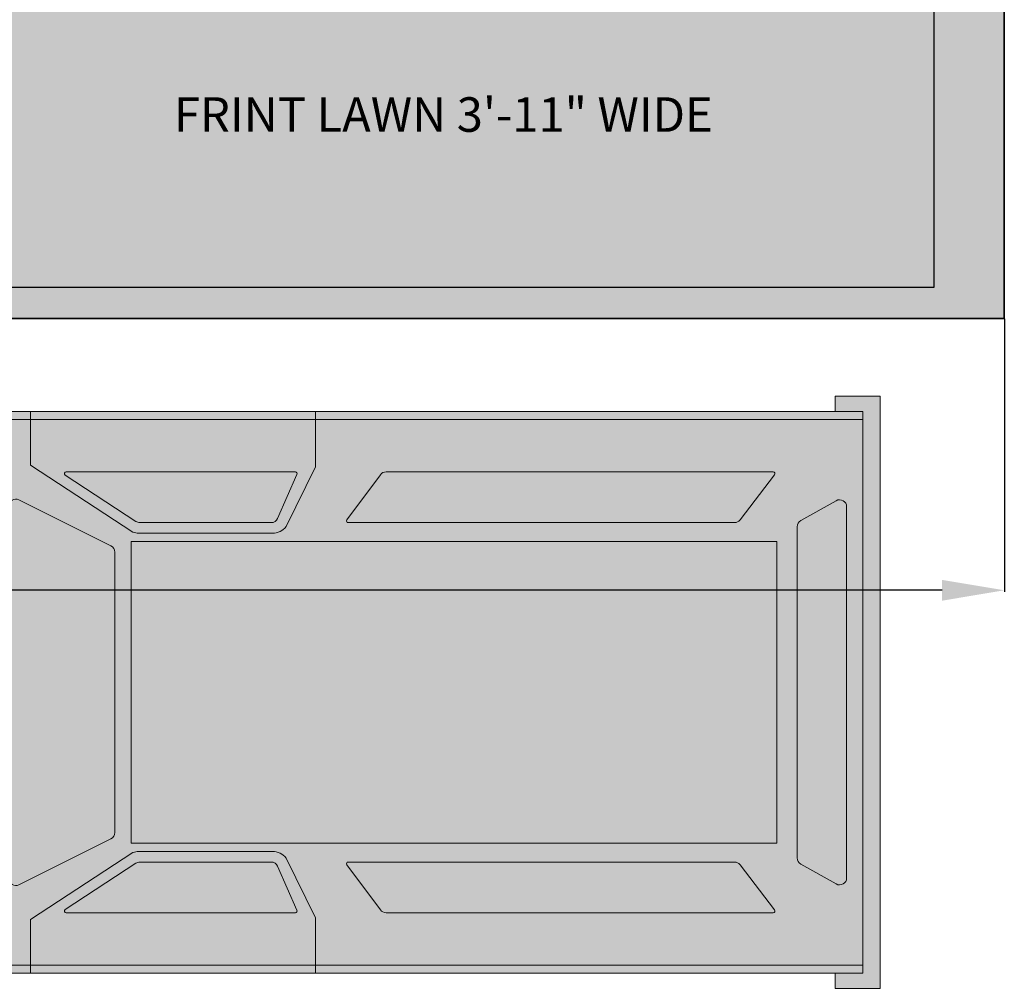
# Model space of a CAD drawing. Units: inches. Extents: x 389 to 971, y 148 to 870.
# Tile 5 of 14: x 722 to 848, y 148 to 273. Entities that reach past the tile are written whole.
import ezdxf

# ---------------------------------------------------------------- set-up
doc = ezdxf.new("R2010")
doc.units = ezdxf.units.IN
doc.header["$MEASUREMENT"] = 0
for name, color, linetype, lineweight in [('A-ANNO-DIMS', 2, 'Continuous', 18), ('A-ANNO-TEXT', 7, 'Continuous', 18), ('C-PROP', 7, 'Continuous', 35), ('C-VEHI', 8, 'Continuous', 13), ('L-GRND-BASE-PATT', 8, 'Continuous', 13), ('L-WALL', 7, 'Continuous', 30)]:
    doc.layers.add(name, color=color, linetype=linetype, lineweight=lineweight)
for name, color, linetype, lineweight, true_color in [('A-WALL-PATT', 18, 'Continuous', 13, 0x000000), ('C-VEHI-PATT', 18, 'Continuous', 13, 0x000000), ('L-GRND-PATT', 39, 'Continuous', 13, 0x603913)]:
    doc.layers.add(name, color=color, linetype=linetype, lineweight=lineweight, true_color=true_color)
doc.styles.get("Standard").update_dxf_attribs({"font": 'arial.ttf'})
doc.dimstyles.get("Standard").update_dxf_attribs({"dimtxt": 8, "dimasz": 8, "dimexe": 0.18, "dimexo": 0.0625, "dimgap": 0.09, "dimtad": 0, "dimtih": 1, "dimtoh": 1, "dimdec": 0, "dimzin": 0, "dimdsep": 46, "dimlunit": 3, "dimtxsty": 'Standard', "dimcen": 0.09, "dimadec": 0, "dimazin": 0, "dimtfac": 1, "dimtdec": 0, "dimtofl": 0, "dimtmove": 0, "dimatfit": 3, "dimfxl": 1, "dimtolj": 1, "dimtzin": 0, "dimarcsym": 0})

# ---------------------------------------------------------------- blocks, each defined once
blk = doc.blocks.new('*U17')
for p, q in [((1.28, 38.87), (175.66, 38.87)), ((1.28, 28.15), (52.13, 28.15)), ((1.28, -28.15), (52.13, -28.15)), ((1.28, -38.87), (175.66, -38.87))]:
    blk.add_line(p, q)
for points in [[(5.57, 40.01), (5.57, 42.18), (0, 42.18), (0, -42.18), (5.57, -42.18), (5.57, -40.01), (1.28, -40.01), (1.28, 40.01)], [(171.74, 40.01), (175.66, 40.01), (175.66, -40.01), (171.74, -40.01), (171.74, -42.18), (178.14, -42.18), (178.14, 42.18), (171.74, 42.18)], [(1.28, 40.01), (175.66, 40.01), (175.66, -40.01), (1.28, -40.01)], [(71.47, 21.48), (163.42, 21.48), (163.42, -21.48), (71.47, -21.48)]]:
    blk.add_lwpolyline(points, close=True)
for points in [[(57.15, 40.01), (57.15, 32.39), (71.72, 22.83, 0.086577), (72.56, 22.68), (91.59, 22.68, 0.227875), (93.54, 23.62), (97.72, 32.11), (97.72, 40.01)], [(57.15, -40.01), (57.15, -32.39), (71.72, -22.83, -0.086577), (72.56, -22.68), (91.59, -22.68, -0.227875), (93.54, -23.62), (97.72, -32.11), (97.72, -40.01)]]:
    blk.add_lwpolyline(points, format="xyb")
for points in [[(62.08, 30.95), (72.14, 24.35, 0.146139), (72.69, 24.18), (91.42, 24.18, 0.29766), (92.33, 24.78), (95.09, 31.05, 0.541236), (94.86, 31.41), (62.21, 31.41, 0.744989)], [(102.19, 24.58), (106.97, 31, -0.236929), (107.78, 31.41), (162.91, 31.41, -0.621576), (163.11, 31), (158.19, 24.58, -0.233368), (157.39, 24.18), (102.39, 24.18, -0.616908)], [(55.49, 27.42), (68.59, 20.89, -0.284287), (69.14, 19.99), (69.14, -19.99, -0.284287), (68.59, -20.89), (55.49, -27.42, -0.557284), (54.05, -26.53), (54.05, 26.53, -0.557284)], [(171.88, 27.31), (166.83, 24.47, 0.271143), (166.32, 23.6), (166.32, -23.6, 0.271143), (166.83, -24.47), (171.88, -27.31, 0.573387), (173.37, -26.44), (173.37, 26.44, 0.573387)], [(62.08, -30.95), (72.14, -24.35, -0.146139), (72.69, -24.18), (91.42, -24.18, -0.29766), (92.33, -24.78), (95.09, -31.05, -0.541236), (94.86, -31.41), (62.21, -31.41, -0.744989)], [(102.19, -24.58), (106.97, -31, 0.236929), (107.78, -31.41), (162.91, -31.41, 0.621576), (163.11, -31), (158.19, -24.58, 0.233368), (157.39, -24.18), (102.39, -24.18, 0.616908)]]:
    blk.add_lwpolyline(points, format="xyb", close=True)
blk = doc.blocks.new('*D44')
at = {"layer": 'A-ANNO-DIMS', "color": 0, "lineweight": -2, "transparency": 16777216}
for p, q in [((428.22, 234.58), (428.22, 199.5)), ((848.22, 234.58), (848.22, 199.5)), ((436.22, 199.68), (629.14, 199.68)), ((840.22, 199.68), (647.29, 199.68))]:
    blk.add_line(p, q, dxfattribs=at)
at = {"layer": 'A-ANNO-DIMS', "color": 0, "transparency": 16777216}
for points in [[(436.22, 201.01), (436.22, 198.34), (428.22, 199.68)], [(840.22, 201.01), (840.22, 198.34), (848.22, 199.68)]]:
    blk.add_solid(points, dxfattribs=at)
at = {"layer": 'Defpoints', "color": 0, "transparency": 16777216}
for p in [(428.22, 234.64), (848.22, 234.64), (848.22, 199.68)]:
    blk.add_point(p, dxfattribs=at)
at = {"layer": 'A-ANNO-DIMS', "color": 0, "transparency": 16777216, "insert": (638.22, 199.68), "char_height": 8, "attachment_point": 5}
blk.add_mtext('\\A1;420', dxfattribs=at)

msp = doc.modelspace()

# ---------------------------------------------------------------- hatches: boundary and pattern name
at = {"layer": 'A-WALL-PATT'}
h = msp.add_hatch(color=256, dxfattribs=at)
h.dxf.hatch_style = 1
h.paths.add_polyline_path([(432.216, 434.6445), (436.3673, 434.6445), (436.3673, 443.6445), (432.216, 443.6445), (432.216, 830.6445), (746.216, 830.6445), (746.216, 823.8175), (755.216, 823.8175), (755.216, 825.6445), (839.216, 825.6445), (839.216, 803.5176), (839.216, 741.6445), (755.216, 741.6445), (755.216, 748.4596), (755.1859, 748.4596), (750.716, 748.4596), (746.216, 748.4596), (746.216, 732.6445), (839.216, 732.6445), (839.216, 600.6445), (708.5171, 600.6445), (708.5171, 596.1445), (708.5171, 591.6445), (794.216, 591.6445), (794.216, 587.4291), (803.216, 587.4291), (803.216, 591.6445), (839.216, 591.6445), (839.216, 466.6012), (803.216, 466.6012), (803.216, 471.0309), (794.216, 471.0309), (794.216, 466.6012), (784.6145, 466.6012), (784.6145, 457.6012), (839.216, 457.6012), (839.216, 447.6445), (839.216, 294.6445), (810.0514, 294.6445), (810.0514, 285.6445), (839.216, 285.6445), (839.216, 238.6445), (590.216, 238.6445), (590.216, 234.6445), (848.216, 234.6445), (848.216, 834.6445), (428.216, 834.6445), (428.216, 234.6445), (437.216, 234.6445), (437.216, 243.6445), (432.216, 243.6445)])
at = {"layer": 'C-VEHI-PATT'}
h = msp.add_hatch(color=256, dxfattribs=at)
h.dxf.hatch_style = 1
h.paths.add_polyline_path([(720.2545, 210.4982), (720.2545, 162.6111, 0.55728405), (721.56, 161.8036), (733.3797, 167.7021, 0.28428722), (733.8792, 168.5096), (733.8792, 204.5997, 0.28428722), (733.3797, 205.4073), (721.56, 211.3058, 0.55728405)], flags=16)
h.paths.add_polyline_path([(672.6289, 151.4772), (723.0515, 151.4772), (723.0515, 157.3254), (736.2011, 165.949, -0.08657677), (736.9651, 166.0823), (754.137, 166.0823, -0.22787473), (755.899, 165.2353), (759.6746, 157.5735), (759.6746, 151.4772), (830.0078, 151.4772), (830.0078, 221.6321), (759.6746, 221.6321), (759.6746, 215.5358), (755.899, 207.8741, -0.22787473), (754.137, 207.0271), (736.9651, 207.0271, -0.08657677), (736.2011, 207.1603), (723.0515, 215.784), (723.0515, 221.6321), (672.6289, 221.6321)])
h.paths.add_polyline_path([(672.6289, 150.445), (676.5048, 150.445), (676.5048, 148.491), (671.4773, 148.491), (671.4773, 224.6184), (676.5048, 224.6184), (676.5048, 222.6644), (672.6289, 222.6644)])
h.paths.add_polyline_path([(735.9785, 205.941), (818.9627, 205.941), (818.9627, 167.1683), (735.9785, 167.1683)], flags=16)
h.paths.add_polyline_path([(727.5014, 158.6254), (736.5823, 164.5807, -0.14613934), (737.0772, 164.7285), (753.9813, 164.7285, -0.29765964), (754.8077, 164.1887), (757.2923, 158.5274, -0.54123619), (757.0857, 158.2111), (727.6252, 158.2111, -0.74498852)], flags=17)
h.paths.add_polyline_path([(727.5014, 214.4839, -0.74498852), (727.6252, 214.8982), (757.0857, 214.8982, -0.54123619), (757.2923, 214.5819), (754.8077, 208.9206, -0.29765964), (753.9813, 208.3808), (737.0772, 208.3808, -0.14613934), (736.5823, 208.5286)], flags=17)
h = msp.add_hatch(color=256, dxfattribs=at)
h.dxf.hatch_style = 1
h.paths.add_polyline_path([(672.6289, 184.5547), (672.6289, 151.4772), (723.0515, 151.4772), (723.0515, 157.3254), (736.2011, 165.949, -0.08657677), (736.9651, 166.0823), (754.137, 166.0823, -0.22787473), (755.899, 165.2353), (759.6746, 157.5735), (759.6746, 151.4772), (830.0078, 151.4772), (830.0078, 221.6321), (759.6746, 221.6321), (759.6746, 215.5358), (755.899, 207.8741, -0.22787473), (754.137, 207.0271), (736.9651, 207.0271, -0.08657677), (736.2011, 207.1603), (723.0515, 215.784), (723.0515, 221.6321), (672.6289, 221.6321), (672.6289, 188.5547), (720.2545, 188.5547), (720.2545, 210.4982, -0.55728405), (721.56, 211.3058), (733.3797, 205.4073, -0.28428722), (733.8792, 204.5997), (733.8792, 168.5096, -0.28428722), (733.3797, 167.7021), (721.56, 161.8036, -0.55728405), (720.2545, 162.6111), (720.2545, 184.5547)], flags=17)
h.paths.add_polyline_path([(672.6289, 151.4772), (723.0515, 151.4772), (723.0515, 157.3254), (736.2011, 165.949, -0.08657677), (736.9651, 166.0823), (754.137, 166.0823, -0.22787473), (755.899, 165.2353), (759.6746, 157.5735), (759.6746, 151.4772), (830.0078, 151.4772), (830.0078, 221.6321), (759.6746, 221.6321), (759.6746, 215.5358), (755.899, 207.8741, -0.22787473), (754.137, 207.0271), (736.9651, 207.0271, -0.08657677), (736.2011, 207.1603), (723.0515, 215.784), (723.0515, 221.6321), (672.6289, 221.6321)], flags=17)
h.paths.add_polyline_path([(672.6289, 150.445), (676.5048, 150.445), (676.5048, 148.491), (671.4773, 148.491), (671.4773, 224.6184), (676.5048, 224.6184), (676.5048, 222.6644), (672.6289, 222.6644)])
h.paths.add_polyline_path([(720.2545, 210.4982, -0.55728405), (721.56, 211.3058), (733.3797, 205.4073, -0.28428722), (733.8792, 204.5997), (733.8792, 168.5096, -0.28428722), (733.3797, 167.7021), (721.56, 161.8036, -0.55728405), (720.2545, 162.6111)], flags=0)
h.paths.add_polyline_path([(727.5014, 158.6254), (736.5823, 164.5807, -0.14613934), (737.0772, 164.7285), (753.9813, 164.7285, -0.29765964), (754.8077, 164.1887), (757.2923, 158.5274, -0.54123619), (757.0857, 158.2111), (727.6252, 158.2111, -0.74498852)], flags=0)
h = msp.add_hatch(color=256, dxfattribs=at)
h.dxf.hatch_style = 1
h.paths.add_polyline_path([(832.2495, 148.491), (832.2495, 224.6184), (826.4762, 224.6184), (826.4762, 222.6644), (830.0078, 222.6644), (830.0078, 150.445), (826.4762, 150.445), (826.4762, 148.491)])
h = msp.add_hatch(color=256, dxfattribs=at)
h.dxf.hatch_style = 1
h.paths.add_polyline_path([(723.0515, 221.6321), (723.0515, 215.784), (736.2011, 207.1603, 0.08657677), (736.9651, 207.0271), (754.137, 207.0271, 0.22787473), (755.899, 207.8741), (759.6746, 215.5358), (759.6746, 221.6321)], flags=16)
h.paths.add_polyline_path([(672.6289, 222.6644), (672.6289, 151.4772), (723.0515, 151.4772), (723.0515, 157.3254), (736.2011, 165.949, -0.08657677), (736.9651, 166.0823), (754.137, 166.0823, -0.22787473), (755.899, 165.2353), (759.6746, 157.5735), (759.6746, 151.4772), (830.0078, 151.4772), (830.0078, 222.6644)])
h = msp.add_hatch(color=256, dxfattribs=at)
h.dxf.hatch_style = 1
h.paths.add_polyline_path([(723.0515, 221.6321), (723.0515, 222.6644), (672.6289, 222.6644), (672.6289, 221.6321)])
h = msp.add_hatch(color=256, dxfattribs=at)
h.dxf.hatch_style = 1
h.paths.add_polyline_path([(723.0515, 222.6644), (723.0515, 221.6321), (759.6746, 221.6321), (759.6746, 222.6644)])
h = msp.add_hatch(color=256, dxfattribs=at)
h.dxf.hatch_style = 1
h.paths.add_polyline_path([(723.0515, 221.6321), (723.0515, 215.784), (736.2011, 207.1603, 0.08657677), (736.9651, 207.0271), (754.137, 207.0271, 0.22787473), (755.899, 207.8741), (759.6746, 215.5358), (759.6746, 221.6321)])
h.paths.add_polyline_path([(757.0857, 214.8982, -0.54123619), (757.2923, 214.5819), (754.8077, 208.9206, -0.29765964), (753.9813, 208.3808), (737.0772, 208.3808, -0.14613934), (736.5823, 208.5286), (727.5014, 214.4839, -0.74498852), (727.6252, 214.8982)], flags=16)
h = msp.add_hatch(color=256, dxfattribs=at)
h.dxf.hatch_style = 1
h.paths.add_polyline_path([(759.6746, 222.6644), (759.6746, 221.6321), (830.0078, 221.6321), (830.0078, 222.6644)])
h = msp.add_hatch(color=256, dxfattribs=at)
h.dxf.hatch_style = 1
h.paths.add_polyline_path([(753.9813, 208.3808, 0.29765964), (754.8077, 208.9206), (757.2923, 214.5819, 0.54123619), (757.0857, 214.8982), (727.6252, 214.8982, 0.74498852), (727.5014, 214.4839), (736.5823, 208.5286, 0.14613934), (737.0772, 208.3808)])
h = msp.add_hatch(color=256, dxfattribs=at)
h.dxf.hatch_style = 1
h.paths.add_polyline_path([(753.9813, 208.3808, 0.29765964), (754.8077, 208.9206), (757.2923, 214.5819, 0.54123619), (757.0857, 214.8982), (727.6252, 214.8982, 0.74498852), (727.5014, 214.4839), (736.5823, 208.5286, 0.14613934), (737.0772, 208.3808)])
h = msp.add_hatch(color=256, dxfattribs=at)
h.dxf.hatch_style = 1
h.paths.add_polyline_path([(813.5241, 208.3808, 0.23336833), (814.2405, 208.7344), (818.6847, 214.5354, 0.62157561), (818.5056, 214.8982), (768.7451, 214.8982, 0.23692874), (768.0214, 214.5349), (763.7056, 208.7412, 0.61690802), (763.8865, 208.3808)])
h = msp.add_hatch(color=256, dxfattribs=at)
h.dxf.hatch_style = 1
h.paths.add_polyline_path([(813.5241, 208.3808, 0.23336833), (814.2405, 208.7344), (818.6847, 214.5354, 0.62157561), (818.5056, 214.8982), (768.7451, 214.8982, 0.23692874), (768.0214, 214.5349), (763.7056, 208.7412, 0.61690802), (763.8865, 208.3808)])
h = msp.add_hatch(color=256, dxfattribs=at)
h.dxf.hatch_style = 1
h.paths.add_polyline_path([(733.8792, 204.5997, 0.28428722), (733.3797, 205.4073), (721.56, 211.3058, 0.55728405), (720.2545, 210.4982), (720.2545, 162.6111, 0.55728405), (721.56, 161.8036), (733.3797, 167.7021, 0.28428722), (733.8792, 168.5096)])
h = msp.add_hatch(color=256, dxfattribs=at)
h.dxf.hatch_style = 1
h.paths.add_polyline_path([(720.2545, 162.6111, 0.55728405), (721.56, 161.8036), (733.3797, 167.7021, 0.28428722), (733.8792, 168.5096), (733.8792, 204.5997, 0.28428722), (733.3797, 205.4073), (721.56, 211.3058, 0.55728405), (720.2545, 210.4982)])
h = msp.add_hatch(color=256, dxfattribs=at)
h.dxf.hatch_style = 1
h.paths.add_polyline_path([(733.8792, 204.5997, 0.28428722), (733.3797, 205.4073), (721.56, 211.3058, 0.55728405), (720.2545, 210.4982), (720.2545, 162.6111, 0.55728405), (721.56, 161.8036), (733.3797, 167.7021, 0.28428722), (733.8792, 168.5096)])
h = msp.add_hatch(color=256, dxfattribs=at)
h.dxf.hatch_style = 1
h.paths.add_polyline_path([(827.9463, 210.4153, 0.5733871), (826.6018, 211.2023), (822.0383, 208.6395, 0.271143), (821.5777, 207.8526), (821.5777, 165.2568, 0.271143), (822.0383, 164.4699), (826.6018, 161.9071, 0.5733871), (827.9463, 162.694)])
h = msp.add_hatch(color=256, dxfattribs=at)
h.dxf.hatch_style = 1
h.paths.add_polyline_path([(821.5777, 165.2568, 0.271143), (822.0383, 164.4699), (826.6018, 161.9071, 0.5733871), (827.9463, 162.694), (827.9463, 210.4153, 0.5733871), (826.6018, 211.2023), (822.0383, 208.6395, 0.271143), (821.5777, 207.8526)])
h = msp.add_hatch(color=256, dxfattribs=at)
h.dxf.hatch_style = 1
h.paths.add_polyline_path([(818.9627, 167.1683), (818.9627, 205.941), (735.9785, 205.941), (735.9785, 167.1683)])
h = msp.add_hatch(color=256, dxfattribs=at)
h.dxf.hatch_style = 1
h.paths.add_polyline_path([(818.9627, 167.1683), (818.9627, 205.941), (735.9785, 205.941), (735.9785, 167.1683)])
h = msp.add_hatch(color=256, dxfattribs=at)
h.dxf.hatch_style = 1
h.paths.add_polyline_path([(727.6252, 158.2111), (757.0857, 158.2111, 0.54123619), (757.2923, 158.5274), (754.8077, 164.1887, 0.29765964), (753.9813, 164.7285), (737.0772, 164.7285, 0.14613934), (736.5823, 164.5807), (727.5014, 158.6254, 0.74498852)], flags=16)
h.paths.add_polyline_path([(759.6746, 151.4772), (759.6746, 157.5735), (755.899, 165.2353, 0.22787473), (754.137, 166.0823), (736.9651, 166.0823, 0.08657677), (736.2011, 165.949), (723.0515, 157.3254), (723.0515, 151.4772)])
h = msp.add_hatch(color=256, dxfattribs=at)
h.dxf.hatch_style = 1
h.paths.add_polyline_path([(757.0857, 158.2111, 0.54123619), (757.2923, 158.5274), (754.8077, 164.1887, 0.29765964), (753.9813, 164.7285), (737.0772, 164.7285, 0.14613934), (736.5823, 164.5807), (727.5014, 158.6254, 0.74498852), (727.6252, 158.2111)])
h = msp.add_hatch(color=256, dxfattribs=at)
h.dxf.hatch_style = 1
h.paths.add_polyline_path([(757.0857, 158.2111, 0.54123619), (757.2923, 158.5274), (754.8077, 164.1887, 0.29765964), (753.9813, 164.7285), (737.0772, 164.7285, 0.14613934), (736.5823, 164.5807), (727.5014, 158.6254, 0.74498852), (727.6252, 158.2111)])
h = msp.add_hatch(color=256, dxfattribs=at)
h.dxf.hatch_style = 1
h.paths.add_polyline_path([(818.5056, 158.2111, 0.62157561), (818.6847, 158.5739), (814.2405, 164.3749, 0.23336833), (813.5241, 164.7285), (763.8865, 164.7285, 0.61690802), (763.7056, 164.3681), (768.0214, 158.5745, 0.23692874), (768.7451, 158.2111)])
h = msp.add_hatch(color=256, dxfattribs=at)
h.dxf.hatch_style = 1
h.paths.add_polyline_path([(818.5056, 158.2111, 0.62157561), (818.6847, 158.5739), (814.2405, 164.3749, 0.23336833), (813.5241, 164.7285), (763.8865, 164.7285, 0.61690802), (763.7056, 164.3681), (768.0214, 158.5745, 0.23692874), (768.7451, 158.2111)])
h = msp.add_hatch(color=256, dxfattribs=at)
h.dxf.hatch_style = 1
h.paths.add_polyline_path([(723.0515, 150.445), (723.0515, 151.4772), (672.6289, 151.4772), (672.6289, 150.445)])
h = msp.add_hatch(color=256, dxfattribs=at)
h.dxf.hatch_style = 1
h.paths.add_polyline_path([(759.6746, 150.445), (759.6746, 151.4772), (723.0515, 151.4772), (723.0515, 150.445)])
h = msp.add_hatch(color=256, dxfattribs=at)
h.dxf.hatch_style = 1
h.paths.add_polyline_path([(759.6746, 151.4772), (759.6746, 150.445), (830.0078, 150.445), (830.0078, 151.4772)])
at = {"layer": 'L-GRND-BASE-PATT'}
h = msp.add_hatch(color=256, dxfattribs=at)
h.dxf.hatch_style = 1
edge = h.paths.add_edge_path(flags=16)
edge.add_ellipse((8782.0026, 354.2473), major_axis=(-8296.9493, 0), ratio=0.84230387, start_angle=-0.09022909, end_angle=0.38386678, ccw=False)
edge.add_ellipse((485.0533, 368.2895), major_axis=(-1.1591, 0), ratio=0.84230387, start_angle=0, end_angle=90, ccw=False)
edge.add_line((483.8943, 368.2895), (483.8943, 387.6039))
edge.add_ellipse((485.0533, 387.2466), major_axis=(1.1591, 0), ratio=0.84230387, start_angle=90, end_angle=180, ccw=False)
edge.add_line((485.0533, 388.2229), (485.5047, 388.2229))
edge.add_ellipse((898.8202, 372.4897), major_axis=(413.7374, 0), ratio=0.84230387, start_angle=176.349572, end_angle=177.82005, ccw=False)
edge.add_ellipse((535.9119, 196.3855), major_axis=(-245.3972, 0), ratio=0.84230387, start_angle=-77.874034, end_angle=-76.219471, ccw=False)
edge.add_ellipse((535.9119, 201.7547), major_axis=(239.1274, 0), ratio=0.84230387, start_angle=100.209539, end_angle=102.444627, ccw=False)
edge.add_ellipse((473.3139, 564.9222), major_axis=(196.5637, 0), ratio=0.84230387, start_angle=-80.743434, end_angle=-77.445067)
edge.add_line((509.5535, 402.1941), (514.3535, 404.8483))
edge.add_line((514.3535, 404.8483), (514.3535, 404.7972))
edge.add_ellipse((514.3535, 404.2644), major_axis=(0.5795, 0), ratio=0.84230387, start_angle=52.06687, end_angle=90, ccw=False)
edge.add_line((514.6716, 404.6725), (519.1535, 402.1941))
edge.add_ellipse((555.3932, 564.9222), major_axis=(-196.5637, 0), ratio=0.84230387, start_angle=77.445067, end_angle=80.743434)
edge.add_ellipse((492.7951, 201.7547), major_axis=(239.1274, 0), ratio=0.84230387, start_angle=77.555373, end_angle=79.790461, ccw=False)
edge.add_ellipse((492.7951, 196.3855), major_axis=(245.3972, 0), ratio=0.84230387, start_angle=76.219471, end_angle=77.874034, ccw=False)
edge.add_ellipse((129.8868, 372.4897), major_axis=(-413.7374, 0), ratio=0.84230387, start_angle=182.17995, end_angle=183.650428, ccw=False)
edge.add_line((543.2023, 388.2229), (544.0779, 388.2229))
edge.add_ellipse((543.6537, 387.2466), major_axis=(-1.1591, 0), ratio=0.84230387, start_angle=180, end_angle=270, ccw=False)
edge.add_line((544.8128, 387.2466), (544.8128, 367.9322))
edge.add_ellipse((543.6537, 368.2895), major_axis=(1.1591, 0), ratio=0.84230387, start_angle=270, end_angle=360, ccw=False)
edge.add_ellipse((-7753.2956, 354.2473), major_axis=(-8296.9493, 0), ratio=0.84230387, start_angle=179.61613322, end_angle=180.09022909, ccw=False)
edge.add_line((543.3912, 298.6608), (544.0779, 298.6608))
edge.add_ellipse((543.6537, 297.6845), major_axis=(1.1591, 0), ratio=0.84230387, start_angle=0, end_angle=90, ccw=False)
edge.add_line((544.8128, 297.6845), (544.8128, 278.3701))
edge.add_ellipse((543.6537, 278.7275), major_axis=(-1.1591, 0), ratio=0.84230387, start_angle=90, end_angle=180, ccw=False)
edge.add_line((543.6537, 277.7512), (543.1566, 277.7512))
edge.add_ellipse((-7753.2956, 354.2473), major_axis=(-8296.9493, 0), ratio=0.84230387, start_angle=179.3813568, end_angle=179.47172853, ccw=False)
edge.add_ellipse((542.4236, 263.2763), major_axis=(-1.7386, 0), ratio=0.84230387, start_angle=179.371763, end_angle=248.464757, ccw=False)
edge.add_ellipse((-7753.8751, 354.2473), major_axis=(-8298.7403, 0), ratio=0.842303866, start_angle=179.35344592, end_angle=179.3717628, ccw=False)
edge.add_ellipse((540.0116, 260.6509), major_axis=(-4.1092, 0), ratio=0.84230387, start_angle=90, end_angle=179.353446, ccw=False)
edge.add_line((540.0116, 257.1897), (488.6954, 257.1897))
edge.add_ellipse((488.6954, 260.6509), major_axis=(4.1092, 0), ratio=0.84230387, start_angle=180.646554, end_angle=270, ccw=False)
edge.add_ellipse((8782.5821, 354.2473), major_axis=(-8298.7403, 0), ratio=0.842303872, start_angle=0.62823723, end_angle=0.64655411, ccw=False)
edge.add_ellipse((486.2834, 263.2763), major_axis=(-1.7386, 0), ratio=0.84230387, start_angle=-68.464756, end_angle=0.628237, ccw=False)
edge.add_ellipse((8782.0026, 354.2473), major_axis=(-8296.9493, 0), ratio=0.84230387, start_angle=0.52827147, end_angle=0.6465541, ccw=False)
edge.add_line((485.5504, 277.7512), (484.6291, 277.7512))
edge.add_ellipse((485.0533, 278.7275), major_axis=(-1.1591, 0), ratio=0.84230387, start_angle=0, end_angle=90, ccw=False)
edge.add_line((483.8943, 278.7275), (483.8943, 298.0418))
edge.add_ellipse((485.0533, 297.6845), major_axis=(1.1591, 0), ratio=0.84230387, start_angle=90, end_angle=180, ccw=False)
edge = h.paths.add_edge_path(flags=0)
edge.add_ellipse((8782.0026, 354.2473), major_axis=(-8295.7902, 0), ratio=0.84230387, start_angle=0.05559431, end_angle=0.37776419, ccw=False)
edge.add_line((486.2179, 346.1978), (489.3905, 335.8384))
edge.add_ellipse((3386.0114, 329.7263), major_axis=(-2896.63, 0), ratio=0.84230387, start_angle=-0.1208974, end_angle=0.3640763)
edge.add_line((489.4638, 311.3204), (486.4666, 299.5521))
edge = h.paths.add_edge_path(flags=0)
edge.add_ellipse((514.3535, 391.3731), major_axis=(-115.1513, 0), ratio=0.84230387, start_angle=76.401865, end_angle=103.598135)
edge.add_line((537.3428, 296.3333), (537.3428, 281.5897))
edge.add_ellipse((514.3535, 376.6295), major_axis=(-115.1513, 0), ratio=0.84230387, start_angle=76.401865, end_angle=103.598135, ccw=False)
edge.add_line((491.3643, 281.5897), (491.3643, 296.3333))
edge = h.paths.add_edge_path(flags=0)
edge.add_line((491.3643, 337.0752), (489.653, 349.9016))
edge.add_ellipse((510.1338, 298.7862), major_axis=(64.0481, 0), ratio=0.84230387, start_angle=94.277421, end_angle=111.834954, ccw=False)
edge.add_line((506.1068, 352.6274), (522.6002, 352.6274))
edge.add_ellipse((518.5732, 298.7862), major_axis=(64.0481, 0), ratio=0.84230387, start_angle=68.165046, end_angle=85.722579, ccw=False)
edge.add_line((539.0541, 349.9016), (537.3428, 337.0752))
edge.add_ellipse((516.5462, 287.5825), major_axis=(62.3305, 0), ratio=0.84230387, start_angle=67.208085, end_angle=85.12993)
edge.add_line((521.008, 339.949), (507.699, 339.949))
edge.add_ellipse((512.1609, 287.5825), major_axis=(62.3305, 0), ratio=0.84230387, start_angle=94.87007, end_angle=112.791915)
edge = h.paths.add_edge_path(flags=0)
edge.add_ellipse((493.6824, 273.9439), major_axis=(-2.3182, 0), ratio=0.84230387, start_angle=-90, end_angle=0, ccw=False)
edge.add_line((493.6824, 275.8965), (535.3743, 275.8965))
edge.add_ellipse((535.0246, 273.9439), major_axis=(2.3182, 0), ratio=0.84230387, start_angle=0, end_angle=90, ccw=False)
edge.add_line((537.3428, 273.9439), (537.3428, 258.6983))
edge.add_line((537.3428, 258.6983), (540.5912, 258.6983))
edge.add_ellipse((540.5912, 260.6509), major_axis=(-2.3182, 0), ratio=0.84230387, start_angle=90, end_angle=179.353446)
edge.add_line((540.5912, 258.6983), (487.7691, 258.6983))
edge.add_ellipse((488.1158, 260.6509), major_axis=(2.3182, 0), ratio=0.84230387, start_angle=180.646554, end_angle=270)
edge.add_line((488.1158, 258.6983), (491.3643, 258.6983))
edge.add_line((491.3643, 258.6983), (491.3643, 274.2384))
h.paths.add_polyline_path([(746.1376, 327.3223), (750.14, 327.3223), (750.14, 326.2831), (798.1694, 326.2831), (798.1694, 327.3223), (802.1718, 327.3223), (802.1718, 309.9784, -0.19047621), (746.1376, 309.9784)], flags=16)
h.paths.add_polyline_path([(782.1596, 313.5685), (782.1596, 309.0415, -0.04962821), (766.1498, 309.0415), (766.1498, 313.5685)], flags=0)
h.paths.add_polyline_path([(755.1859, 344.9352), (755.1859, 373.9163), (788.1244, 373.9163), (788.1244, 344.9352)], flags=16)
h.paths.add_polyline_path([(757.1859, 346.9352), (757.1859, 371.9163), (786.1244, 371.9163), (786.1244, 346.9352)], flags=0)
h.paths.add_polyline_path([(803.6446, 338.4879), (803.6446, 342.4903), (804.6838, 342.4903), (804.6838, 390.5197), (803.6446, 390.5197), (803.6446, 394.5221), (820.9885, 394.5221, -0.19047621), (820.9885, 338.4879)], flags=16)
h.paths.add_polyline_path([(806.8707, 326.6963), (806.4254, 327.1416), (806.4724, 326.6297)], flags=16)
h.paths.add_polyline_path([(822.0328, 317.4008), (822.1942, 317.8933), (821.5626, 317.9885)], flags=16)
h.paths.add_polyline_path([(817.3984, 358.5001), (817.3984, 374.5099), (821.9254, 374.5099, -0.04962821), (821.9254, 358.5001)], flags=0)
h.paths.add_polyline_path([(808.1446, 418.9737), (808.2247, 418.5632), (808.5395, 418.5787)], flags=16)
h.paths.add_polyline_path([(820.3159, 412.669), (820.4772, 413.1615), (819.8457, 413.2568)], flags=16)
h.paths.add_polyline_path([(466.3155, 235.5246), (517.3807, 235.5246), (517.3807, 244.4269), (466.3155, 244.4269)], flags=24)
h.paths.add_polyline_path([(739.8737, 256.2), (815.404, 256.2), (815.404, 265.3454), (739.8737, 265.3454)], flags=24)
h.paths.add_polyline_path([(750.6082, 393.6667), (791.5681, 393.6667), (791.5681, 412.3933), (750.6082, 412.3933)], flags=24)
h.paths.add_polyline_path([(438.9631, 410.0619), (484.6204, 410.0619), (484.6204, 429.1217), (438.9631, 429.1217)], flags=24)
edge = h.paths.add_edge_path()
edge.add_line((839.216, 285.6445), (611.8787, 285.6445))
edge.add_line((611.8787, 285.6445), (604.387, 285.6445))
edge.add_line((604.387, 285.6445), (595.387, 285.6445))
edge.add_line((595.387, 285.6445), (595.387, 370.1554))
edge.add_line((595.387, 370.1554), (604.0817, 370.1554))
edge.add_line((604.0817, 370.1554), (604.0817, 371.3788))
edge.add_line((604.0817, 371.3788), (632.0195, 371.3788))
edge.add_arc((604.0817, 370.1554), 27.9645, 2.507491, 90)
edge.add_line((604.0817, 398.1199), (599.887, 398.1652))
edge.add_line((599.887, 398.1652), (604.4225, 398.1652))
edge.add_arc((604.4225, 428.4021), 30.2369, 270, 357.492509)
edge.add_line((634.6305, 427.0792), (604.4225, 427.0792))
edge.add_line((604.4225, 427.0792), (604.4225, 428.4021))
edge.add_line((604.4225, 428.4021), (599.887, 428.4021))
edge.add_line((599.887, 428.4021), (595.387, 428.4021))
edge.add_line((595.387, 428.4021), (595.387, 434.6445))
edge.add_line((595.387, 434.6445), (585.0791, 434.6445))
edge.add_line((585.0791, 434.6445), (540.3922, 434.6445))
edge.add_line((540.3922, 434.6445), (526.7125, 434.6445))
edge.add_line((526.7125, 434.6445), (488.4095, 434.6445))
edge.add_line((488.4095, 434.6445), (432.216, 434.6445))
edge.add_line((432.216, 434.6445), (432.216, 243.6445))
edge.add_line((432.216, 243.6445), (437.216, 243.6445))
edge.add_line((437.216, 243.6445), (437.216, 234.6445))
edge.add_line((437.216, 234.6445), (581.216, 234.6445))
edge.add_line((581.216, 234.6445), (581.216, 238.6445))
edge.add_line((581.216, 238.6445), (581.216, 243.6445))
edge.add_line((581.216, 243.6445), (590.216, 243.6445))
edge.add_line((590.216, 243.6445), (590.216, 238.6445))
edge.add_line((590.216, 238.6445), (839.216, 238.6445))
edge.add_line((839.216, 238.6445), (839.216, 285.6445))
at = {"layer": 'L-GRND-PATT'}
h = msp.add_hatch(dxfattribs=at)
h.set_pattern_fill('EARTH', color=256, angle=45)
h.set_pattern_definition([(45, (0, 0), (0, 8.980256), [6.35, -6.35]), (45, (-1.684, 1.684), (0, 8.980256), [6.35, -6.35]), (45, (-3.3676, 3.3676), (0, 8.980256), [6.35, -6.35]), (135, (-3.3676, 4.49), (-8.980256, 0), [6.35, -6.35]), (135, (-1.684, 6.174), (-8.980256, 0), [6.35, -6.35]), (135, (0, 7.858), (-8.980256, 0), [6.35, -6.35])])
h.paths.add_polyline_path([(432.216, 243.6445), (437.216, 243.6445), (437.216, 234.6445), (581.216, 234.6445), (581.216, 238.6445), (581.216, 243.6445), (590.216, 243.6445), (590.216, 238.6445), (839.216, 238.6445), (839.216, 285.6445), (810.0514, 285.6445), (733.8057, 285.6445), (684.2434, 285.6445), (611.8787, 285.6445), (604.387, 285.6445), (595.387, 285.6445), (595.387, 370.1554), (604.0817, 370.1554), (604.0817, 371.3788), (632.0195, 371.3788, 0.40145271), (604.0817, 398.1199), (599.887, 398.1652), (604.4225, 398.1652, 0.40145271), (634.6305, 427.0792), (604.4225, 427.0792), (604.4225, 428.4021), (599.887, 428.4021), (595.387, 428.4021), (595.387, 434.6445), (585.0791, 434.6445), (540.3922, 434.6445), (526.7125, 434.6445), (488.4095, 434.6445), (432.216, 434.6445)])
edge = h.paths.add_edge_path(flags=16)
edge.add_line((483.8943, 278.7275), (483.8943, 298.2564))
edge.add_ellipse((485.0533, 297.6845), major_axis=(1.1591, 0), ratio=0.84230387, start_angle=90, end_angle=180, ccw=False)
edge.add_ellipse((8782.0026, 354.2473), major_axis=(-8296.9493, 0), ratio=0.84230387, start_angle=-0.09022909, end_angle=0.38386678, ccw=False)
edge.add_ellipse((485.0533, 368.2895), major_axis=(-1.1591, 0), ratio=0.84230387, start_angle=0, end_angle=90, ccw=False)
edge.add_line((483.8943, 368.2895), (483.8943, 387.8185))
edge.add_ellipse((485.0533, 387.2466), major_axis=(1.1591, 0), ratio=0.84230387, start_angle=90, end_angle=180, ccw=False)
edge.add_ellipse((898.8202, 372.4897), major_axis=(413.7374, 0), ratio=0.84230387, start_angle=176.349572, end_angle=177.82005, ccw=False)
edge.add_ellipse((535.9119, 196.3855), major_axis=(-245.3972, 0), ratio=0.84230387, start_angle=-77.874034, end_angle=-76.219471, ccw=False)
edge.add_ellipse((535.9119, 201.7547), major_axis=(239.1274, 0), ratio=0.84230387, start_angle=100.209539, end_angle=102.444627, ccw=False)
edge.add_ellipse((473.3139, 564.9222), major_axis=(196.5637, 0), ratio=0.84230387, start_angle=-80.743434, end_angle=-77.445067)
edge.add_line((509.5535, 402.1941), (514.3535, 404.8483))
edge.add_line((514.3535, 404.8483), (519.1535, 402.1941))
edge.add_ellipse((555.3932, 564.9222), major_axis=(-196.5637, 0), ratio=0.84230387, start_angle=77.445067, end_angle=80.743434)
edge.add_ellipse((492.7951, 201.7547), major_axis=(239.1274, 0), ratio=0.84230387, start_angle=77.555373, end_angle=79.790461, ccw=False)
edge.add_ellipse((492.7951, 196.3855), major_axis=(245.3972, 0), ratio=0.84230387, start_angle=76.219471, end_angle=77.874034, ccw=False)
edge.add_ellipse((129.8868, 372.4897), major_axis=(-413.7374, 0), ratio=0.84230387, start_angle=182.17995, end_angle=183.650428, ccw=False)
edge.add_line((543.2023, 388.2229), (544.3327, 388.2229))
edge.add_ellipse((543.6537, 387.2466), major_axis=(-1.1591, 0), ratio=0.84230387, start_angle=180, end_angle=270, ccw=False)
edge.add_line((544.8128, 387.2466), (544.8128, 367.7176))
edge.add_ellipse((543.6537, 368.2895), major_axis=(1.1591, 0), ratio=0.84230387, start_angle=270, end_angle=360, ccw=False)
edge.add_ellipse((-7753.2956, 354.2473), major_axis=(-8296.9493, 0), ratio=0.84230387, start_angle=179.61613322, end_angle=180.09022909, ccw=False)
edge.add_ellipse((543.6537, 297.6845), major_axis=(1.1591, 0), ratio=0.84230387, start_angle=0, end_angle=90, ccw=False)
edge.add_line((544.8128, 297.6845), (544.8128, 278.1556))
edge.add_ellipse((543.6537, 278.7275), major_axis=(-1.1591, 0), ratio=0.84230387, start_angle=90, end_angle=180, ccw=False)
edge.add_ellipse((-7753.2956, 354.2473), major_axis=(-8296.9493, 0), ratio=0.84230387, start_angle=179.3813568, end_angle=179.47172853, ccw=False)
edge.add_ellipse((542.4236, 263.2763), major_axis=(-1.7386, 0), ratio=0.84230387, start_angle=179.371763, end_angle=248.464757, ccw=False)
edge.add_ellipse((-7753.8751, 354.2473), major_axis=(-8298.7403, 0), ratio=0.842303866, start_angle=179.35344592, end_angle=179.3717628, ccw=False)
edge.add_ellipse((540.0116, 260.6509), major_axis=(-4.1092, 0), ratio=0.84230387, start_angle=90, end_angle=179.353446, ccw=False)
edge.add_line((540.0116, 257.1897), (488.0808, 257.1897))
edge.add_ellipse((488.6954, 260.6509), major_axis=(4.1092, 0), ratio=0.84230387, start_angle=180.646554, end_angle=270, ccw=False)
edge.add_ellipse((8782.5821, 354.2473), major_axis=(-8298.7403, 0), ratio=0.842303872, start_angle=0.62823723, end_angle=0.64655411, ccw=False)
edge.add_ellipse((486.2834, 263.2763), major_axis=(-1.7386, 0), ratio=0.84230387, start_angle=-68.464756, end_angle=0.628237, ccw=False)
edge.add_ellipse((8782.0026, 354.2473), major_axis=(-8296.9493, 0), ratio=0.84230387, start_angle=0.52827147, end_angle=0.6465541, ccw=False)
edge.add_line((485.5504, 277.7512), (484.3744, 277.7512))
edge.add_ellipse((485.0533, 278.7275), major_axis=(-1.1591, 0), ratio=0.84230387, start_angle=0, end_angle=90, ccw=False)
edge = h.paths.add_edge_path(flags=0)
edge.add_ellipse((488.1158, 260.6509), major_axis=(2.3182, 0), ratio=0.84230387, start_angle=180.646554, end_angle=270)
edge.add_line((488.1158, 258.6983), (491.3643, 258.6983))
edge.add_line((491.3643, 258.6983), (491.3643, 274.4686))
edge.add_ellipse((493.6824, 273.9439), major_axis=(-2.3182, 0), ratio=0.84230387, start_angle=-90, end_angle=0, ccw=False)
edge.add_line((493.6824, 275.8965), (535.6476, 275.8965))
edge.add_ellipse((535.0246, 273.9439), major_axis=(2.3182, 0), ratio=0.84230387, start_angle=0, end_angle=90, ccw=False)
edge.add_line((537.3428, 273.9439), (537.3428, 258.6983))
edge.add_line((537.3428, 258.6983), (541.2086, 258.6983))
edge.add_ellipse((540.5912, 260.6509), major_axis=(-2.3182, 0), ratio=0.84230387, start_angle=90, end_angle=179.353446, ccw=False)
edge.add_line((540.5912, 258.6983), (487.4984, 258.6983))
edge = h.paths.add_edge_path(flags=0)
edge.add_line((491.3643, 281.5897), (491.3643, 296.3333))
edge.add_ellipse((514.3535, 391.3731), major_axis=(-115.1513, 0), ratio=0.84230387, start_angle=76.401865, end_angle=103.598135)
edge.add_line((537.3428, 296.3333), (537.3428, 281.5897))
edge.add_ellipse((514.3535, 376.6295), major_axis=(-115.1513, 0), ratio=0.84230387, start_angle=76.401865, end_angle=103.598135, ccw=False)
edge = h.paths.add_edge_path(flags=0)
edge.add_ellipse((8782.0026, 354.2473), major_axis=(-8295.7902, 0), ratio=0.84230387, start_angle=0.05559431, end_angle=0.37776419, ccw=False)
edge.add_line((486.2179, 346.1978), (489.3905, 335.8384))
edge.add_ellipse((3386.0114, 329.7263), major_axis=(-2896.63, 0), ratio=0.84230387, start_angle=-0.1208974, end_angle=0.3640763)
edge.add_line((489.4638, 311.3204), (486.4666, 299.5521))
edge = h.paths.add_edge_path(flags=0)
edge.add_line((491.3643, 337.0752), (489.653, 349.9016))
edge.add_ellipse((510.1338, 298.7862), major_axis=(64.0481, 0), ratio=0.84230387, start_angle=94.277421, end_angle=111.834954, ccw=False)
edge.add_line((506.1068, 352.6274), (522.6002, 352.6274))
edge.add_ellipse((518.5732, 298.7862), major_axis=(64.0481, 0), ratio=0.84230387, start_angle=68.165046, end_angle=85.722579, ccw=False)
edge.add_line((539.0541, 349.9016), (537.3428, 337.0752))
edge.add_ellipse((516.5462, 287.5825), major_axis=(62.3305, 0), ratio=0.84230387, start_angle=67.208085, end_angle=85.12993)
edge.add_line((521.008, 339.949), (507.699, 339.949))
edge.add_ellipse((512.1609, 287.5825), major_axis=(62.3305, 0), ratio=0.84230387, start_angle=94.87007, end_angle=112.791915)
h.paths.add_polyline_path([(466.3155, 235.5246), (517.3807, 235.5246), (517.3807, 244.4269), (466.3155, 244.4269)], flags=24)
h.paths.add_polyline_path([(739.8737, 256.2), (815.404, 256.2), (815.404, 265.3454), (739.8737, 265.3454)], flags=24)
h.paths.add_polyline_path([(438.9631, 410.0619), (484.6204, 410.0619), (484.6204, 429.1217), (438.9631, 429.1217)], flags=24)

# ---------------------------------------------------------------- linework, layer by layer
at = {"layer": 'C-PROP'}
for p, q in [((848.216, 234.6445), (848.216, 834.6445)), ((428.216, 234.6445), (848.216, 234.6445))]:
    msp.add_line(p, q, dxfattribs=at)
at = {"layer": 'L-WALL'}
for p, q in [((839.216, 238.6445), (839.216, 285.6445)), ((590.216, 238.6445), (839.216, 238.6445))]:
    msp.add_line(p, q, dxfattribs=at)

# ---------------------------------------------------------------- block references
at = {"layer": 'C-VEHI', "xscale": 0.902504869863545, "yscale": 0.902504869863545, "zscale": 0.902504869863545}
msp.add_blockref('*U17', (671.4773, 186.5547), dxfattribs=at)

# ---------------------------------------------------------------- texts
at = {"layer": 'A-ANNO-TEXT', "insert": (741.4918, 263.0795), "char_height": 4.437973, "attachment_point": 1}
msp.add_mtext_dynamic_manual_height_columns('FRINT LAWN 3\'-11" WIDE', width=100.723064, gutter_width=22.1899, heights=[0], dxfattribs=at)

# ---------------------------------------------------------------- dimensions: what is measured, and where the dimension line sits
at = {"layer": 'A-ANNO-DIMS'}
dim = msp.add_linear_dim(base=(848.216, 199.6753), p1=(428.216, 234.6445), p2=(848.216, 234.6445), dimstyle='Standard', override={"dimdec": 0, "dimlfac": 1, "dimrnd": 0, "dimzin": 0, "dimdsep": 46, "dimlunit": 2}, dxfattribs=at)
dim.commit()
dim.dimension.update_dxf_attribs({"geometry": '*D44', "text_midpoint": (638.216, 199.6753)})

doc.saveas('drawing.dxf')
